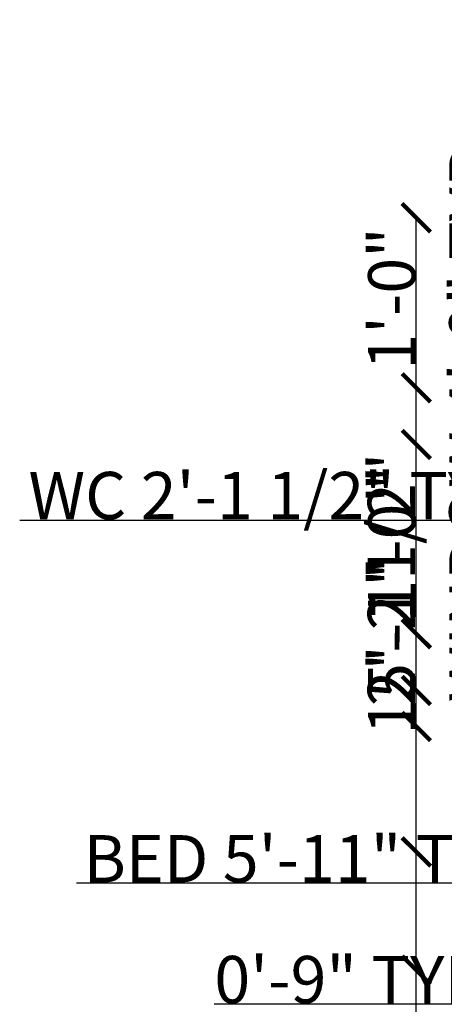
# Model space of a CAD drawing. Units: inches. Extents: x 1957 to 2456, y 1504 to 2088.
# Tile 2 of 6: x 1957 to 2047, y 1703 to 1911. Entities that reach past the tile are written whole.
import ezdxf

# ---------------------------------------------------------------- set-up
doc = ezdxf.new("R2010")
doc.units = ezdxf.units.IN
doc.header["$LTSCALE"] = 2
doc.layers.add('A-ANNO-DIMS', color=2, linetype='Continuous', lineweight=18)
doc.styles.get("Standard").update_dxf_attribs({"font": 'arial.ttf'})
doc.dimstyles.get("Standard").update_dxf_attribs({"dimtxt": 10, "dimasz": 6, "dimexe": 0.18, "dimexo": 0.0625, "dimgap": 0.09, "dimtad": 1, "dimdec": 1, "dimzin": 0, "dimdsep": 46, "dimlunit": 4, "dimtxsty": 'Standard', "dimblk": 'ARCHTICK', "dimcen": 0.09, "dimse1": 1, "dimse2": 1, "dimadec": 0, "dimazin": 0, "dimtfac": 1, "dimtdec": 1, "dimtofl": 0, "dimtmove": 0, "dimatfit": 3, "dimfxl": 1, "dimtolj": 1, "dimtzin": 0, "dimarcsym": 0})

# ---------------------------------------------------------------- blocks, each defined once
blk = doc.blocks.new('_ArchTick')
at = {"color": 0, "linetype": 'ByBlock', "const_width": 0.15}
blk.add_lwpolyline([(-0.5, -0.5), (0.5, 0.5)], dxfattribs=at)
blk = doc.blocks.new('*D23')
at = {"layer": 'A-ANNO-DIMS', "color": 0, "lineweight": -2, "transparency": 16777216}
for p, q in [((2057.83, 1758.05), (2057.83, 1890.77)), ((2057.83, 1710.05), (2057.83, 1758.05))]:
    blk.add_line(p, q, dxfattribs=at)
at = {"layer": 'Defpoints', "color": 0, "transparency": 16777216}
for p in [(2057.83, 1758.05), (2065.03, 1758.05), (2065.03, 1710.05)]:
    blk.add_point(p, dxfattribs=at)
at = {"layer": 'A-ANNO-DIMS', "color": 0, "lineweight": -2, "transparency": 16777216, "xscale": 6, "yscale": 6, "zscale": 6}
for p, rotation in [((2057.83, 1758.05), 90), ((2057.83, 1710.05), 270)]:
    blk.add_blockref('_ArchTick', p, dxfattribs=dict(at, rotation=rotation))
at = {"layer": 'A-ANNO-DIMS', "color": 0, "transparency": 16777216, "insert": (2052.57, 1827.41), "char_height": 10, "attachment_point": 5, "rotation": 90}
blk.add_mtext('\\A1;WINDOW 4\'-0" TYP.', dxfattribs=at)
blk = doc.blocks.new('*D24')
at = {"layer": 'A-ANNO-DIMS', "color": 0, "lineweight": -2, "transparency": 16777216}
for p, q in [((2065.03, 1702.85), (1997.9, 1702.85)), ((2074.03, 1702.85), (2065.03, 1702.85))]:
    blk.add_line(p, q, dxfattribs=at)
at = {"layer": 'Defpoints', "color": 0, "transparency": 16777216}
for p in [(2065.03, 1710.05), (2074.03, 1710.05), (2065.03, 1702.85)]:
    blk.add_point(p, dxfattribs=at)
at = {"layer": 'A-ANNO-DIMS', "color": 0, "lineweight": -2, "transparency": 16777216, "xscale": 6, "yscale": 6, "zscale": 6}
for p, rotation in [((2065.03, 1702.85), 179.9999999999986), ((2074.03, 1702.85), 359.9999999999986)]:
    blk.add_blockref('_ArchTick', p, dxfattribs=dict(at, rotation=rotation))
at = {"layer": 'A-ANNO-DIMS', "color": 0, "transparency": 16777216, "insert": (2028.47, 1708.05), "char_height": 10, "attachment_point": 5}
blk.add_mtext('\\A1;0\'-9" TYP.', dxfattribs=at)
blk = doc.blocks.new('*D27')
at = {"layer": 'A-ANNO-DIMS', "color": 0, "lineweight": -2, "transparency": 16777216}
for p, q in [((2077.63, 1857.22), (2077.63, 2031.19)), ((2077.63, 1833.22), (2077.63, 1857.22))]:
    blk.add_line(p, q, dxfattribs=at)
at = {"layer": 'Defpoints', "color": 0, "transparency": 16777216}
for p in [(2074.03, 1857.22), (2077.63, 1857.22), (2074.03, 1833.22)]:
    blk.add_point(p, dxfattribs=at)
at = {"layer": 'A-ANNO-DIMS', "color": 0, "lineweight": -2, "transparency": 16777216, "xscale": 6, "yscale": 6, "zscale": 6}
for p, rotation in [((2077.63, 1857.22), 90), ((2077.63, 1833.22), 270)]:
    blk.add_blockref('_ArchTick', p, dxfattribs=dict(at, rotation=rotation))
at = {"layer": 'A-ANNO-DIMS', "color": 0, "transparency": 16777216, "insert": (2072.37, 1947.2), "char_height": 10, "attachment_point": 5, "rotation": 90}
blk.add_mtext('\\A1;VENT WINDOW 2\'-0" TYP.', dxfattribs=at)
blk = doc.blocks.new('*D29')
at = {"layer": 'A-ANNO-DIMS', "color": 0, "lineweight": -2, "transparency": 16777216}
for p, q in [((2075.86, 1728.42), (1968.79, 1728.42)), ((2146.9, 1728.42), (2075.86, 1728.42))]:
    blk.add_line(p, q, dxfattribs=at)
at = {"layer": 'Defpoints', "color": 0, "transparency": 16777216}
for p in [(2075.86, 1728.42), (2075.86, 1717.76), (2146.9, 1717.76)]:
    blk.add_point(p, dxfattribs=at)
at = {"layer": 'A-ANNO-DIMS', "color": 0, "lineweight": -2, "transparency": 16777216, "xscale": 6, "yscale": 6, "zscale": 6, "rotation": 180}
blk.add_blockref('_ArchTick', (2075.86, 1728.42), dxfattribs=at)
at = {"layer": 'A-ANNO-DIMS', "color": 0, "lineweight": -2, "transparency": 16777216, "xscale": 6, "yscale": 6, "zscale": 6}
blk.add_blockref('_ArchTick', (2146.9, 1728.42), dxfattribs=at)
at = {"layer": 'A-ANNO-DIMS', "color": 0, "transparency": 16777216, "insert": (2019.32, 1733.61), "char_height": 10, "attachment_point": 5}
blk.add_mtext('\\A1;BED 5\'-11" TYP.', dxfattribs=at)
blk = doc.blocks.new('*D33')
at = {"layer": 'A-ANNO-DIMS', "color": 0, "lineweight": -2, "transparency": 16777216}
for p, q in [((2074.82, 1805.18), (1956.82, 1805.18)), ((2100.26, 1805.18), (2074.82, 1805.18))]:
    blk.add_line(p, q, dxfattribs=at)
at = {"layer": 'Defpoints', "color": 0, "transparency": 16777216}
for p in [(2074.82, 1805.18), (2074.82, 1801.36), (2100.26, 1801.36)]:
    blk.add_point(p, dxfattribs=at)
at = {"layer": 'A-ANNO-DIMS', "color": 0, "lineweight": -2, "transparency": 16777216, "xscale": 6, "yscale": 6, "zscale": 6, "rotation": 180}
blk.add_blockref('_ArchTick', (2074.82, 1805.18), dxfattribs=at)
at = {"layer": 'A-ANNO-DIMS', "color": 0, "lineweight": -2, "transparency": 16777216, "xscale": 6, "yscale": 6, "zscale": 6}
blk.add_blockref('_ArchTick', (2100.26, 1805.18), dxfattribs=at)
at = {"layer": 'A-ANNO-DIMS', "color": 0, "transparency": 16777216, "insert": (2012.82, 1810.44), "char_height": 10, "attachment_point": 5}
blk.add_mtext('\\A1;WC 2\'-1 1/2" TYP.', dxfattribs=at)
blk = doc.blocks.new('*D52')
at = {"layer": 'A-ANNO-DIMS', "color": 0, "lineweight": -2, "transparency": 16777216}
blk.add_line((2040.63, 1610.22), (2040.63, 1710.05), dxfattribs=at)
at = {"layer": 'Defpoints', "color": 0, "transparency": 16777216}
for p in [(2040.63, 1710.05), (2074.03, 1710.05), (2074.03, 1610.22)]:
    blk.add_point(p, dxfattribs=at)
at = {"layer": 'A-ANNO-DIMS', "color": 0, "lineweight": -2, "transparency": 16777216, "xscale": 6, "yscale": 6, "zscale": 6}
for p, rotation in [((2040.63, 1710.05), 90), ((2040.63, 1610.22), 270)]:
    blk.add_blockref('_ArchTick', p, dxfattribs=dict(at, rotation=rotation))
at = {"layer": 'A-ANNO-DIMS', "color": 0, "transparency": 16777216, "insert": (2035.44, 1660.14), "char_height": 10, "attachment_point": 5, "rotation": 90}
blk.add_mtext('\\A1;8\'-4"', dxfattribs=at)
blk = doc.blocks.new('*D56')
at = {"layer": 'A-ANNO-DIMS', "color": 0, "lineweight": -2, "transparency": 16777216}
blk.add_line((2040.63, 1688.22), (2040.63, 1869.22), dxfattribs=at)
at = {"layer": 'Defpoints', "color": 0, "transparency": 16777216}
for p in [(2040.63, 1869.22), (2367.03, 1869.22), (2367.03, 1688.22)]:
    blk.add_point(p, dxfattribs=at)
at = {"layer": 'A-ANNO-DIMS', "color": 0, "lineweight": -2, "transparency": 16777216, "xscale": 6, "yscale": 6, "zscale": 6}
for p, rotation in [((2040.63, 1869.22), 90), ((2040.63, 1688.22), 270)]:
    blk.add_blockref('_ArchTick', p, dxfattribs=dict(at, rotation=rotation))
at = {"layer": 'A-ANNO-DIMS', "color": 0, "transparency": 16777216, "insert": (2035.44, 1778.72), "char_height": 10, "attachment_point": 5, "rotation": 90}
blk.add_mtext('\\A1;15\'-1"', dxfattribs=at)
blk = doc.blocks.new('*D57')
at = {"layer": 'A-ANNO-DIMS', "color": 0, "lineweight": -2, "transparency": 16777216}
for p, q in [((2040.63, 1781.22), (2040.63, 1813.04)), ((2040.63, 1769.22), (2040.63, 1781.22))]:
    blk.add_line(p, q, dxfattribs=at)
at = {"layer": 'Defpoints', "color": 0, "transparency": 16777216}
for p in [(2040.63, 1781.22), (2074.03, 1781.22), (2074.03, 1769.22)]:
    blk.add_point(p, dxfattribs=at)
at = {"layer": 'A-ANNO-DIMS', "color": 0, "lineweight": -2, "transparency": 16777216, "xscale": 6, "yscale": 6, "zscale": 6}
for p, rotation in [((2040.63, 1781.22), 90), ((2040.63, 1769.22), 270)]:
    blk.add_blockref('_ArchTick', p, dxfattribs=dict(at, rotation=rotation))
at = {"layer": 'A-ANNO-DIMS', "color": 0, "transparency": 16777216, "insert": (2035.44, 1800.13), "char_height": 10, "attachment_point": 5, "rotation": 90}
blk.add_mtext('\\A1;1\'-0"', dxfattribs=at)
blk = doc.blocks.new('*D58')
at = {"layer": 'A-ANNO-DIMS', "color": 0, "lineweight": -2, "transparency": 16777216}
for p, q in [((2040.63, 1833.22), (2040.63, 1865.04)), ((2040.63, 1821.22), (2040.63, 1833.22))]:
    blk.add_line(p, q, dxfattribs=at)
at = {"layer": 'Defpoints', "color": 0, "transparency": 16777216}
for p in [(2040.63, 1833.22), (2074.03, 1833.22), (2074.03, 1821.22)]:
    blk.add_point(p, dxfattribs=at)
at = {"layer": 'A-ANNO-DIMS', "color": 0, "lineweight": -2, "transparency": 16777216, "xscale": 6, "yscale": 6, "zscale": 6}
for p, rotation in [((2040.63, 1833.22), 90), ((2040.63, 1821.22), 270)]:
    blk.add_blockref('_ArchTick', p, dxfattribs=dict(at, rotation=rotation))
at = {"layer": 'A-ANNO-DIMS', "color": 0, "transparency": 16777216, "insert": (2035.44, 1852.13), "char_height": 10, "attachment_point": 5, "rotation": 90}
blk.add_mtext('\\A1;1\'-0"', dxfattribs=at)
blk = doc.blocks.new('*D67')
at = {"layer": 'A-ANNO-DIMS', "color": 0, "lineweight": -2, "transparency": 16777216}
for p, q in [((2040.63, 1761.57), (2040.63, 1817.8)), ((2040.63, 1735.04), (2040.63, 1761.57))]:
    blk.add_line(p, q, dxfattribs=at)
at = {"layer": 'Defpoints', "color": 0, "transparency": 16777216}
for p in [(2040.63, 1761.57), (2287.11, 1761.57), (2287.11, 1735.04)]:
    blk.add_point(p, dxfattribs=at)
at = {"layer": 'A-ANNO-DIMS', "color": 0, "lineweight": -2, "transparency": 16777216, "xscale": 6, "yscale": 6, "zscale": 6}
for p, rotation in [((2040.63, 1761.57), 90), ((2040.63, 1735.04), 270)]:
    blk.add_blockref('_ArchTick', p, dxfattribs=dict(at, rotation=rotation))
at = {"layer": 'A-ANNO-DIMS', "color": 0, "transparency": 16777216, "insert": (2035.37, 1792.69), "char_height": 10, "attachment_point": 5, "rotation": 90}
blk.add_mtext('\\A1;2\'-2 1/2"', dxfattribs=at)

msp = doc.modelspace()

# ---------------------------------------------------------------- dimensions: what is measured, and where the dimension line sits
at = {"layer": 'A-ANNO-DIMS'}
for base, p1, p2, angle, text, picture, middle in [((2077.63, 1857.22), (2074.03, 1833.22), (2074.03, 1857.22), 90, 'VENT WINDOW <> TYP.', '*D27', (2072.37, 1947.2)), ((2057.83, 1758.05), (2065.03, 1710.05), (2065.03, 1758.05), 90, 'WINDOW <> TYP.', '*D23', (2052.57, 1827.41)), ((2074.82, 1805.18), (2100.26, 1801.36), (2074.82, 1801.36), 180, 'WC <> TYP.', '*D33', (2012.82, 1810.44)), ((2075.86, 1728.42), (2146.9, 1717.76), (2075.86, 1717.76), 180, 'BED <> TYP.', '*D29', (2019.32, 1733.61)), ((2065.03, 1702.85), (2074.03, 1710.05), (2065.03, 1710.05), 180, '<> TYP.', '*D24', (2028.47, 1708.05))]:
    dim = msp.add_linear_dim(base=base, p1=p1, p2=p2, angle=angle, text=text, dimstyle='Standard', override={"dimdec": 1, "dimlfac": 1, "dimrnd": 0, "dimzin": 1, "dimdsep": 46, "dimlunit": 4, "dimfrac": 2}, dxfattribs=at)
    dim.commit()
    dim.dimension.update_dxf_attribs({"geometry": picture, "text_midpoint": middle})
for base, p1, p2, picture, middle in [((2040.63, 1869.22), (2367.03, 1688.22), (2367.03, 1869.22), '*D56', (2035.44, 1778.72)), ((2040.63, 1833.22), (2074.03, 1821.22), (2074.03, 1833.22), '*D58', (2035.44, 1852.13)), ((2040.63, 1761.57), (2287.11, 1735.04), (2287.11, 1761.57), '*D67', (2035.37, 1792.69)), ((2040.63, 1781.22), (2074.03, 1769.22), (2074.03, 1781.22), '*D57', (2035.44, 1800.13)), ((2040.63, 1710.05), (2074.03, 1610.22), (2074.03, 1710.05), '*D52', (2035.44, 1660.14))]:
    dim = msp.add_linear_dim(base=base, p1=p1, p2=p2, angle=90, dimstyle='Standard', override={"dimdec": 1, "dimlfac": 1, "dimrnd": 0, "dimzin": 1, "dimdsep": 46, "dimlunit": 4, "dimfrac": 2}, dxfattribs=at)
    dim.commit()
    dim.dimension.update_dxf_attribs({"geometry": picture, "text_midpoint": middle})

doc.saveas('drawing.dxf')
